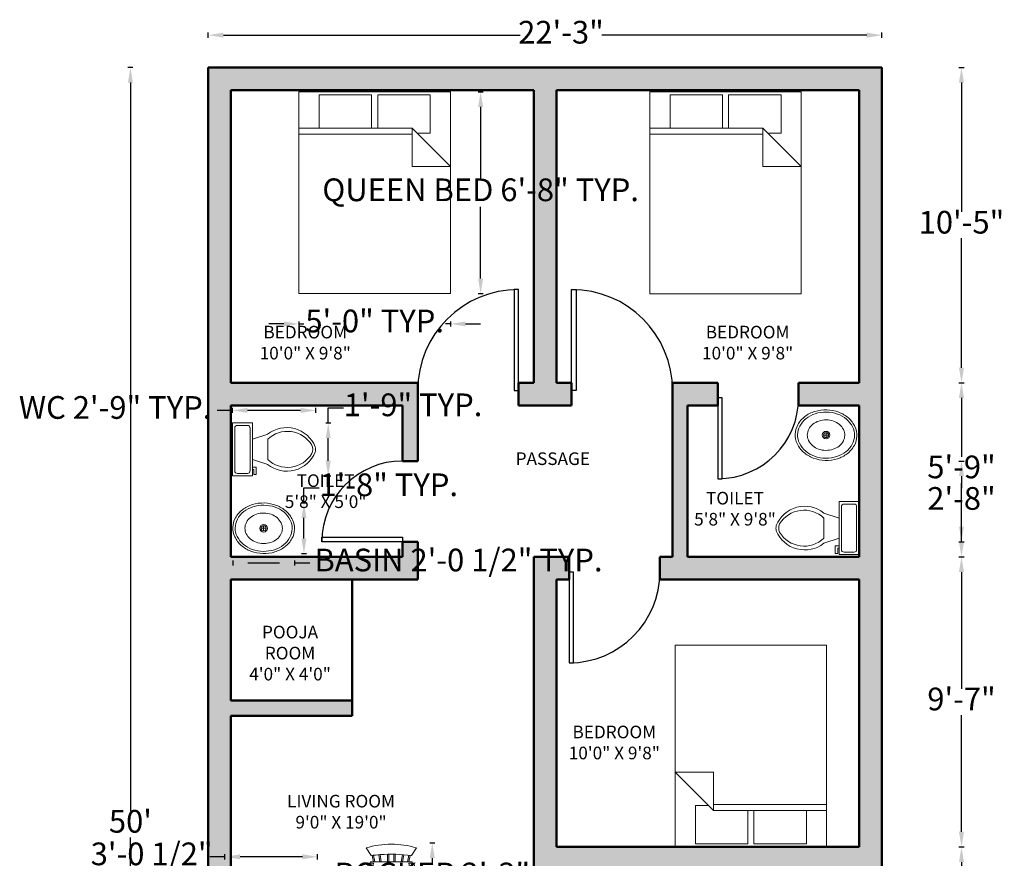
# Model space of a CAD drawing. Units: inches. Extents: x -31 to 401, y -19 to 637.
# Tile 2 of 2: x -31 to 359, y 305 to 637. Entities that reach past the tile are written whole.
import ezdxf

# ---------------------------------------------------------------- set-up
doc = ezdxf.new("R2010")
doc.units = ezdxf.units.IN
for name, color, linetype, lineweight in [('A-ANNO-DIMS', 2, 'Continuous', 18), ('A-AREA-IDEN', 7, 'Continuous', 25), ('A-DOOR', 4, 'Continuous', 25), ('A-FLOR-FIXT', 9, 'Continuous', 18), ('A-FURN', 8, 'Continuous', 18), ('A-WALL', 7, 'Continuous', 50), ('A-WALL-PATT', 252, 'Continuous', 13)]:
    doc.layers.add(name, color=color, linetype=linetype, lineweight=lineweight)
doc.styles.get("Standard").update_dxf_attribs({"font": 'arial.ttf'})
doc.dimstyles.new('ISO-25', dxfattribs={"dimtxt": 9, "dimasz": 6, "dimexe": 1, "dimexo": 2, "dimtad": 0, "dimtih": 1, "dimtoh": 1, "dimdec": 1, "dimlunit": 3, "dimtxsty": 'Standard', "dimcen": 2.5, "dimadec": 0, "dimazin": 0, "dimtfac": 1, "dimtdec": 1, "dimtmove": 0, "dimatfit": 3, "dimfxl": 1, "dimfxlon": 1, "dimarcsym": 0})

# ---------------------------------------------------------------- blocks, each defined once
blk = doc.blocks.new('*U6')
for p, q in [((0, 0), (0, 6)), ((36, 0), (36, 6))]:
    blk.add_line(p, q)
blk.add_lwpolyline([(0, 0), (0, -36), (1.75, -36), (1.75, 0)], close=True)
blk.add_arc((0, 0), 36, 270, 0)
blk = doc.blocks.new('*U4')
for p, q in [((0, 0), (0, -6)), ((-40, 0), (-40, -6))]:
    blk.add_line(p, q)
blk.add_lwpolyline([(0, 0), (0, 40), (-1.75, 40), (-1.75, 0)], close=True)
blk.add_arc((0, 0), 40, 90, 180)
blk = doc.blocks.new('*U10')
for p, q in [((0, 0), (0, -6)), ((32, 0), (32, -6))]:
    blk.add_line(p, q)
blk.add_lwpolyline([(0, 0), (0, 32), (1.75, 32), (1.75, 0)], close=True)
blk.add_arc((0, 0), 32, 0, 90)
blk = doc.blocks.new('*U3')
for p, q in [((0, 0), (0, -6)), ((40, 0), (40, -6))]:
    blk.add_line(p, q)
blk.add_lwpolyline([(0, 0), (0, 40), (1.75, 40), (1.75, 0)], close=True)
blk.add_arc((0, 0), 40, 0, 90)
blk = doc.blocks.new('*U5')
for p, q in [((0, 0), (0, 6)), ((32, 0), (32, 6))]:
    blk.add_line(p, q)
blk.add_lwpolyline([(0, 0), (0, -32), (1.75, -32), (1.75, 0)], close=True)
blk.add_arc((0, 0), 32, 270, 0)
blk = doc.blocks.new('Bed - Queen')
for p, q in [((0, -80.00003), (0, 0)), ((0, 0), (59.99999, 0)), ((59.99999, 0), (59.99999, -80.00003)), ((7.99999, -1.2), (28.79998, -1.2)), ((7.99999, -14.4), (7.99999, -1.2)), ((28.79998, -1.2), (28.79998, -14.4)), ((31.19999, -1.2), (51.99999, -1.2)), ((31.19999, -14.4), (31.19999, -1.2)), ((51.99999, -1.2), (51.99999, -16.4)), ((0, -14.4), (44.8, -14.4)), ((59.99999, -29.6), (44.8, -14.4)), ((44.8, -14.4), (44.8, -29.6)), ((44.8, -16.8), (0, -16.8)), ((51.99999, -16.4), (46.79936, -16.4)), ((44.8, -29.6), (59.99999, -29.6)), ((59.99999, -80.00003), (0, -80.00003))]:
    blk.add_line(p, q)
blk = doc.blocks.new('Chair - Rocking')
for p, q in [((-8, -4.5), (-10, -1.5)), ((8, -4.5), (10, -1.5)), ((-9, -7.5), (-12, -18.49999)), ((-7, -7.5), (-9, -7.5)), ((-9, -18.49999), (-7, -7.5)), ((-8.23428, -6.99939), (-8.3093, -7.47958)), ((-8.23041, -7), (8.23915, -7)), ((-7.5, -4.5), (-7, -7)), ((-6.5, -7), (-7.02225, -4.43)), ((-4.5, -7), (-4.96674, -4.19951)), ((-4, -7), (-4.40532, -4.16272)), ((-1.5, -4.05012), (-1.5, -7)), ((-1, -7), (-1, -4.05012)), ((1, -7), (1, -4.04655)), ((1.5, -4.05012), (1.5, -7)), ((4, -7), (4.40187, -4.18694)), ((4.5, -7), (4.96761, -4.19437)), ((6.5, -7), (7, -4.4057)), ((7.5, -4.5), (7, -7)), ((7, -7.5), (9, -7.5)), ((9, -18.49999), (7, -7.5)), ((8.31071, -7.48854), (8.23449, -7.00073)), ((9, -7.5), (12, -18.49999)), ((-10.36644, -20.64523), (-10.5, -21.49999)), ((-9, -22.49999), (-9.5, -26.49999)), ((0, -22.49999), (-9.5, -22.49999)), ((-8, -26.49999), (-7.5, -22.49999)), ((0, -22.49999), (9.5, -22.49999)), ((8, -26.49999), (7.5, -22.49999)), ((9, -22.49999), (9.5, -26.49999)), ((10.5, -21.49999), (10.3575, -20.58798)), ((-9.5, -26.49999), (-8, -26.49999)), ((9.5, -26.49999), (8, -26.49999))]:
    blk.add_line(p, q)
for centre, radius, start, end in [((0, -34.08333), 34.08333, 72.93847, 107.0615), ((0, -68.25004), 64.25, 93.92211, 97.15267), ((0, -68.25004), 64.25, 82.84733, 93.92211), ((-10.5, -18.99999), 1.58114, 161.5651, 18.43495), ((10.5, -18.99999), 1.58114, 161.5651, 18.43495), ((-9.5, -21.49999), 1, 180, 270), ((9.5, -21.49999), 1, 270, 0)]:
    blk.add_arc(centre, radius, start, end)
blk = doc.blocks.new('Toilet - top')
for p, q in [((9.5, -6), (9.5, -2)), ((-10, -8.5), (-8, -8.5)), ((-10, -9.5), (-10, -8.5)), ((-7, -9.5), (-10, -9.5)), ((-8, -8.5), (-8, -8)), ((-7, -8), (-7, -9.5)), ((-4, -8), (-6, -14)), ((4, -8), (6, -14)), ((4, -14), (-4, -14))]:
    blk.add_line(p, q)
blk.add_lwpolyline([(10.5, -8), (10.5, 0), (-10.5, 0), (-10.5, -8)], close=True)
for points in [[(-9.5, -2), (-9.5, -6)], [(8.5, -1), (-8.5, -1)], [(-8.5, -7), (8.5, -7)]]:
    blk.add_lwpolyline(points)
for centre, radius, start, end in [((-8.62, -1.88), 0.884, 81.8699, 188.1301), ((8.62, -1.88), 0.884, 351.8699, 98.1301), ((-8.62, -6.12), 0.884, 171.8699, 278.1301), ((8.62, -6.12), 0.884, 261.8699, 8.1301), ((3.52, -21.58), 12.17, 141.4691, 247.9714), ((4.2, -21.82), 11.33, 136.3677, 238.9468), ((-3.52, -21.58), 12.17, 292.0284, 38.5307), ((-4.2, -21.82), 11.33, 301.053, 43.6321), ((0, -27.88), 4, 245.7318, 294.2682), ((0, -29), 4, 254.8605, 285.1395)]:
    blk.add_arc(centre, radius, start, end)
blk = doc.blocks.new('Sink - Oval top')
for p, q in [((-1, 0), (1, 0)), ((0, 1), (0, -1))]:
    blk.add_line(p, q)
for points in [[(-12.23, 0.39, 0.117634), (-11.46, -3.36, 0.104469), (-8.88, -6.8, 0.090016), (-5.08, -9.07, 0.08192), (-0.32, -10.02, 0.08192), (4.49, -9.38, 0.090016), (8.42, -7.36, 0.104469), (11.22, -4.09, 0.117634), (12.23, -0.39, 0.117634), (11.46, 3.36, 0.104469), (8.88, 6.8, 0.090016), (5.08, 9.07, 0.08192), (0.32, 10.02, 0.08192), (-4.49, 9.38, 0.090016), (-8.42, 7.36, 0.104469), (-11.22, 4.09, 0.117634)], [(-11.29, 0.16, 0.118622), (-10.52, -3.25, 0.104678), (-8.07, -6.36, 0.089562), (-4.54, -8.37, 0.081185), (-0.13, -9.15, 0.081185), (4.3, -8.49, 0.089562), (7.89, -6.58, 0.104678), (10.42, -3.55, 0.118622), (11.29, -0.16, 0.118622), (10.52, 3.25, 0.104678), (8.07, 6.36, 0.089562), (4.54, 8.37, 0.081185), (0.13, 9.15, 0.081185), (-4.3, 8.49, 0.089562), (-7.89, 6.58, 0.104678), (-10.42, 3.55, 0.118622)], [(-7.42, 0.08, 0.118283), (-6.91, -2.17, 0.104607), (-5.29, -4.21, 0.089718), (-2.97, -5.53, 0.081436), (-0.07, -6.04, 0.081436), (2.84, -5.59, 0.089718), (5.2, -4.33, 0.104607), (6.86, -2.32, 0.118283), (7.42, -0.08, 0.118283), (6.91, 2.17, 0.104607), (5.29, 4.21, 0.089718), (2.97, 5.53, 0.081436), (0.07, 6.04, 0.081436), (-2.84, 5.59, 0.089718), (-5.2, 4.33, 0.104607), (-6.86, 2.32, 0.118283)]]:
    blk.add_lwpolyline(points, format="xyb", close=True)
for radius in [1.5, 1]:
    blk.add_circle((0, 0), radius)
blk = doc.blocks.new('*D20')
at = {"layer": 'A-ANNO-DIMS', "color": 0, "lineweight": -2, "transparency": 16777216}
for p, q in [((13.91, 618.38), (11.91, 618.38)), ((12.91, 612.38), (12.91, 323.6)), ((12.91, 24.38), (12.91, 313.16)), ((13.91, 18.38), (11.91, 18.38))]:
    blk.add_line(p, q, dxfattribs=at)
at = {"layer": 'A-ANNO-DIMS', "color": 0, "transparency": 16777216}
for points in [[(11.91, 612.38), (13.91, 612.38), (12.91, 618.38)], [(11.91, 24.38), (13.91, 24.38), (12.91, 18.38)]]:
    blk.add_solid(points, dxfattribs=at)
at = {"layer": 'Defpoints', "color": 0, "transparency": 16777216}
for p in [(43.78, 618.38), (12.91, 18.38), (43.78, 18.38)]:
    blk.add_point(p, dxfattribs=at)
at = {"layer": 'A-ANNO-DIMS', "color": 0, "transparency": 16777216, "insert": (12.91, 318.38), "char_height": 9, "attachment_point": 5}
blk.add_mtext("50'", dxfattribs=at)
blk = doc.blocks.new('*D21')
at = {"layer": 'A-ANNO-DIMS', "color": 0, "lineweight": -2, "transparency": 16777216}
for p, q in [((43.78, 630.2), (43.78, 632.2)), ((49.78, 631.2), (167.43, 631.2)), ((304.78, 631.2), (199.75, 631.2)), ((310.78, 630.2), (310.78, 632.2))]:
    blk.add_line(p, q, dxfattribs=at)
at = {"layer": 'A-ANNO-DIMS', "color": 0, "transparency": 16777216}
for points in [[(49.78, 632.2), (49.78, 630.2), (43.78, 631.2)], [(304.78, 632.2), (304.78, 630.2), (310.78, 631.2)]]:
    blk.add_solid(points, dxfattribs=at)
at = {"layer": 'Defpoints', "color": 0, "transparency": 16777216}
for p in [(310.78, 631.2), (43.78, 618.38), (310.78, 618.38)]:
    blk.add_point(p, dxfattribs=at)
at = {"layer": 'A-ANNO-DIMS', "color": 0, "transparency": 16777216, "insert": (183.59, 631.2), "char_height": 9, "attachment_point": 5}
blk.add_mtext('22\'-3"', dxfattribs=at)
blk = doc.blocks.new('*D22')
at = {"layer": 'A-ANNO-DIMS', "color": 0, "lineweight": -2, "transparency": 16777216}
for p, q in [((150.73, 608.73), (152.73, 608.73)), ((151.73, 602.73), (151.73, 574.28)), ((151.73, 534.73), (151.73, 563.17)), ((150.73, 528.73), (152.73, 528.73))]:
    blk.add_line(p, q, dxfattribs=at)
at = {"layer": 'A-ANNO-DIMS', "color": 0, "transparency": 16777216}
for points in [[(150.73, 602.73), (152.73, 602.73), (151.73, 608.73)], [(150.73, 534.73), (152.73, 534.73), (151.73, 528.73)]]:
    blk.add_solid(points, dxfattribs=at)
at = {"layer": 'Defpoints', "color": 0, "transparency": 16777216}
for p in [(139.73, 608.73), (151.73, 608.73), (139.73, 528.73)]:
    blk.add_point(p, dxfattribs=at)
at = {"layer": 'A-ANNO-DIMS', "color": 0, "transparency": 16777216, "insert": (151.73, 568.73), "char_height": 9, "attachment_point": 5}
blk.add_mtext('QUEEN BED 6\'-8" TYP.', dxfattribs=at)
blk = doc.blocks.new('*D23')
at = {"layer": 'A-ANNO-DIMS', "color": 0, "lineweight": -2, "transparency": 16777216}
for p, q in [((73.73, 516.73), (67.73, 516.73)), ((79.73, 517.73), (79.73, 515.73)), ((79.73, 516.73), (81.67, 516.73)), ((139.73, 516.73), (137.78, 516.73)), ((139.73, 517.73), (139.73, 515.73)), ((145.73, 516.73), (151.73, 516.73))]:
    blk.add_line(p, q, dxfattribs=at)
at = {"layer": 'A-ANNO-DIMS', "color": 0, "transparency": 16777216}
for points in [[(73.73, 517.73), (73.73, 515.73), (79.73, 516.73)], [(145.73, 517.73), (145.73, 515.73), (139.73, 516.73)]]:
    blk.add_solid(points, dxfattribs=at)
at = {"layer": 'Defpoints', "color": 0, "transparency": 16777216}
for p in [(79.73, 528.73), (139.73, 528.73), (139.73, 516.73)]:
    blk.add_point(p, dxfattribs=at)
at = {"layer": 'A-ANNO-DIMS', "color": 0, "transparency": 16777216, "insert": (109.73, 516.73), "char_height": 9, "attachment_point": 5}
blk.add_mtext('5\'-0" TYP.', dxfattribs=at)
blk = doc.blocks.new('*D24')
at = {"layer": 'A-ANNO-DIMS', "color": 0, "lineweight": -2, "transparency": 16777216}
for p, q in [((53.32, 482.44), (47.32, 482.44)), ((53.32, 481.44), (53.32, 483.44)), ((80.36, 482.44), (59.32, 482.44)), ((86.36, 481.44), (86.36, 483.44))]:
    blk.add_line(p, q, dxfattribs=at)
at = {"layer": 'A-ANNO-DIMS', "color": 0, "transparency": 16777216}
for points in [[(59.32, 483.44), (59.32, 481.44), (53.32, 482.44)], [(80.36, 483.44), (80.36, 481.44), (86.36, 482.44)]]:
    blk.add_solid(points, dxfattribs=at)
at = {"layer": 'Defpoints', "color": 0, "transparency": 16777216}
for p in [(53.32, 482.44), (53.32, 477.49), (86.36, 477.49)]:
    blk.add_point(p, dxfattribs=at)
at = {"layer": 'A-ANNO-DIMS', "color": 0, "transparency": 16777216, "insert": (6.86, 482.44), "char_height": 9, "attachment_point": 5}
blk.add_mtext('WC 2\'-9" TYP.', dxfattribs=at)
blk = doc.blocks.new('*D25')
at = {"layer": 'A-ANNO-DIMS', "color": 0, "lineweight": -2, "transparency": 16777216}
for p, q in [((91.32, 477.49), (91.32, 483.49)), ((91.32, 483.49), (97.32, 483.49)), ((90.32, 477.49), (92.32, 477.49)), ((91.32, 462.49), (91.32, 471.49)), ((90.32, 456.49), (92.32, 456.49))]:
    blk.add_line(p, q, dxfattribs=at)
at = {"layer": 'A-ANNO-DIMS', "color": 0, "transparency": 16777216}
for points in [[(90.32, 471.49), (92.32, 471.49), (91.32, 477.49)], [(90.32, 462.49), (92.32, 462.49), (91.32, 456.49)]]:
    blk.add_solid(points, dxfattribs=at)
at = {"layer": 'Defpoints', "color": 0, "transparency": 16777216}
for p in [(86.36, 477.49), (91.32, 477.49), (86.36, 456.49)]:
    blk.add_point(p, dxfattribs=at)
at = {"layer": 'A-ANNO-DIMS', "color": 0, "transparency": 16777216, "insert": (124.95, 483.49), "char_height": 9, "attachment_point": 5}
blk.add_mtext('1\'-9" TYP.', dxfattribs=at)
blk = doc.blocks.new('*D26')
at = {"layer": 'A-ANNO-DIMS', "color": 0, "lineweight": -2, "transparency": 16777216}
for p, q in [((53.46, 422.97), (53.46, 420.97)), ((59.46, 421.97), (72.01, 421.97)), ((78.01, 422.97), (78.01, 420.97)), ((78.01, 421.97), (84.01, 421.97))]:
    blk.add_line(p, q, dxfattribs=at)
at = {"layer": 'A-ANNO-DIMS', "color": 0, "transparency": 16777216}
for points in [[(59.46, 422.97), (59.46, 420.97), (53.46, 421.97)], [(72.01, 422.97), (72.01, 420.97), (78.01, 421.97)]]:
    blk.add_solid(points, dxfattribs=at)
at = {"layer": 'Defpoints', "color": 0, "transparency": 16777216}
for p in [(53.46, 425.65), (78.01, 425.65), (78.01, 421.97)]:
    blk.add_point(p, dxfattribs=at)
at = {"layer": 'A-ANNO-DIMS', "color": 0, "transparency": 16777216, "insert": (142.96, 421.97), "char_height": 9, "attachment_point": 5}
blk.add_mtext('BASIN 2\'-0 1/2" TYP.', dxfattribs=at)
blk = doc.blocks.new('*D27')
at = {"layer": 'A-ANNO-DIMS', "color": 0, "lineweight": -2, "transparency": 16777216}
for p, q in [((81.69, 445.79), (81.69, 451.79)), ((81.69, 451.79), (87.69, 451.79)), ((80.69, 445.79), (82.69, 445.79)), ((81.69, 431.65), (81.69, 439.79)), ((80.69, 425.65), (82.69, 425.65))]:
    blk.add_line(p, q, dxfattribs=at)
at = {"layer": 'A-ANNO-DIMS', "color": 0, "transparency": 16777216}
for points in [[(80.69, 439.79), (82.69, 439.79), (81.69, 445.79)], [(80.69, 431.65), (82.69, 431.65), (81.69, 425.65)]]:
    blk.add_solid(points, dxfattribs=at)
at = {"layer": 'Defpoints', "color": 0, "transparency": 16777216}
for p in [(78.01, 445.79), (81.69, 445.79), (78.01, 425.65)]:
    blk.add_point(p, dxfattribs=at)
at = {"layer": 'A-ANNO-DIMS', "color": 0, "transparency": 16777216, "insert": (115.32, 451.79), "char_height": 9, "attachment_point": 5}
blk.add_mtext('1\'-8" TYP.', dxfattribs=at)
blk = doc.blocks.new('*D29')
at = {"layer": 'A-ANNO-DIMS', "color": 0, "lineweight": -2, "transparency": 16777216}
for p, q in [((50.4, 305.47), (44.4, 305.47)), ((50.4, 304.47), (50.4, 306.47)), ((81.07, 305.47), (56.4, 305.47)), ((87.07, 304.47), (87.07, 306.47))]:
    blk.add_line(p, q, dxfattribs=at)
at = {"layer": 'A-ANNO-DIMS', "color": 0, "transparency": 16777216}
for points in [[(56.4, 306.47), (56.4, 304.47), (50.4, 305.47)], [(81.07, 306.47), (81.07, 304.47), (87.07, 305.47)]]:
    blk.add_solid(points, dxfattribs=at)
at = {"layer": 'Defpoints', "color": 0, "transparency": 16777216}
for p in [(50.4, 305.47), (50.4, 292.87), (87.07, 292.87)]:
    blk.add_point(p, dxfattribs=at)
at = {"layer": 'A-ANNO-DIMS', "color": 0, "transparency": 16777216, "insert": (21.33, 305.47), "char_height": 9, "attachment_point": 5}
blk.add_mtext('3\'-0 1/2"', dxfattribs=at)
blk = doc.blocks.new('*D30')
at = {"layer": 'A-ANNO-DIMS', "color": 0, "lineweight": -2, "transparency": 16777216}
for p, q in [((131.57, 310.98), (133.57, 310.98)), ((132.57, 304.98), (132.57, 302.76)), ((132.57, 289.98), (132.57, 292.19)), ((131.57, 283.98), (133.57, 283.98))]:
    blk.add_line(p, q, dxfattribs=at)
at = {"layer": 'A-ANNO-DIMS', "color": 0, "transparency": 16777216}
for points in [[(131.57, 304.98), (133.57, 304.98), (132.57, 310.98)], [(131.57, 289.98), (133.57, 289.98), (132.57, 283.98)]]:
    blk.add_solid(points, dxfattribs=at)
at = {"layer": 'Defpoints', "color": 0, "transparency": 16777216}
for p in [(128.52, 310.98), (132.57, 310.98), (128.52, 283.98)]:
    blk.add_point(p, dxfattribs=at)
at = {"layer": 'A-ANNO-DIMS', "color": 0, "transparency": 16777216, "insert": (132.57, 297.48), "char_height": 9, "attachment_point": 5}
blk.add_mtext('ROCKER 2\'-3"', dxfattribs=at)
blk = doc.blocks.new('*D45')
at = {"layer": 'A-ANNO-DIMS', "color": 0, "lineweight": -2, "transparency": 16777216}
for p, q in [((341.33, 309.38), (343.33, 309.38)), ((342.33, 303.38), (342.33, 238.1)), ((342.33, 162.38), (342.33, 227.66)), ((341.33, 156.38), (343.33, 156.38))]:
    blk.add_line(p, q, dxfattribs=at)
at = {"layer": 'A-ANNO-DIMS', "color": 0, "transparency": 16777216}
for points in [[(341.33, 303.38), (343.33, 303.38), (342.33, 309.38)], [(341.33, 162.38), (343.33, 162.38), (342.33, 156.38)]]:
    blk.add_solid(points, dxfattribs=at)
at = {"layer": 'Defpoints', "color": 0, "transparency": 16777216}
for p in [(301.78, 309.38), (342.33, 309.38), (301.78, 156.38)]:
    blk.add_point(p, dxfattribs=at)
at = {"layer": 'A-ANNO-DIMS', "color": 0, "transparency": 16777216, "insert": (342.33, 232.88), "char_height": 9, "attachment_point": 5}
blk.add_mtext('12\'-9"', dxfattribs=at)
blk = doc.blocks.new('*D46')
at = {"layer": 'A-ANNO-DIMS', "color": 0, "lineweight": -2, "transparency": 16777216}
for p, q in [((341.33, 424.38), (343.33, 424.38)), ((342.33, 418.38), (342.33, 372.1)), ((342.33, 315.38), (342.33, 361.66)), ((341.33, 309.38), (343.33, 309.38))]:
    blk.add_line(p, q, dxfattribs=at)
at = {"layer": 'A-ANNO-DIMS', "color": 0, "transparency": 16777216}
for points in [[(341.33, 418.38), (343.33, 418.38), (342.33, 424.38)], [(341.33, 315.38), (343.33, 315.38), (342.33, 309.38)]]:
    blk.add_solid(points, dxfattribs=at)
at = {"layer": 'Defpoints', "color": 0, "transparency": 16777216}
for p in [(301.78, 424.38), (342.33, 424.38), (301.78, 309.38)]:
    blk.add_point(p, dxfattribs=at)
at = {"layer": 'A-ANNO-DIMS', "color": 0, "transparency": 16777216, "insert": (342.33, 366.88), "char_height": 9, "attachment_point": 5}
blk.add_mtext('9\'-7"', dxfattribs=at)
blk = doc.blocks.new('*D47')
at = {"layer": 'A-ANNO-DIMS', "color": 0, "lineweight": -2, "transparency": 16777216}
for p, q in [((341.33, 493.38), (343.33, 493.38)), ((342.33, 487.38), (342.33, 464.1)), ((342.33, 430.38), (342.33, 453.66)), ((341.33, 424.38), (343.33, 424.38))]:
    blk.add_line(p, q, dxfattribs=at)
at = {"layer": 'A-ANNO-DIMS', "color": 0, "transparency": 16777216}
for points in [[(341.33, 487.38), (343.33, 487.38), (342.33, 493.38)], [(341.33, 430.38), (343.33, 430.38), (342.33, 424.38)]]:
    blk.add_solid(points, dxfattribs=at)
at = {"layer": 'Defpoints', "color": 0, "transparency": 16777216}
for p in [(301.78, 493.38), (342.33, 493.38), (301.78, 424.38)]:
    blk.add_point(p, dxfattribs=at)
at = {"layer": 'A-ANNO-DIMS', "color": 0, "transparency": 16777216, "insert": (342.33, 458.88), "char_height": 9, "attachment_point": 5}
blk.add_mtext('5\'-9"', dxfattribs=at)
blk = doc.blocks.new('*D48')
at = {"layer": 'A-ANNO-DIMS', "color": 0, "lineweight": -2, "transparency": 16777216}
for p, q in [((341.33, 618.38), (343.33, 618.38)), ((342.33, 612.38), (342.33, 561.1)), ((342.33, 499.38), (342.33, 550.66)), ((341.33, 493.38), (343.33, 493.38))]:
    blk.add_line(p, q, dxfattribs=at)
at = {"layer": 'A-ANNO-DIMS', "color": 0, "transparency": 16777216}
for points in [[(341.33, 612.38), (343.33, 612.38), (342.33, 618.38)], [(341.33, 499.38), (343.33, 499.38), (342.33, 493.38)]]:
    blk.add_solid(points, dxfattribs=at)
at = {"layer": 'Defpoints', "color": 0, "transparency": 16777216}
for p in [(310.78, 618.38), (342.33, 618.38), (301.78, 493.38)]:
    blk.add_point(p, dxfattribs=at)
at = {"layer": 'A-ANNO-DIMS', "color": 0, "transparency": 16777216, "insert": (342.33, 555.88), "char_height": 9, "attachment_point": 5}
blk.add_mtext('10\'-5"', dxfattribs=at)
blk = doc.blocks.new('*D49')
at = {"layer": 'A-ANNO-DIMS', "color": 0, "lineweight": -2, "transparency": 16777216}
for p, q in [((341.33, 462.38), (343.33, 462.38)), ((342.33, 456.38), (342.33, 451.6)), ((342.33, 436.38), (342.33, 441.16)), ((341.33, 430.38), (343.33, 430.38))]:
    blk.add_line(p, q, dxfattribs=at)
at = {"layer": 'A-ANNO-DIMS', "color": 0, "transparency": 16777216}
for points in [[(341.33, 456.38), (343.33, 456.38), (342.33, 462.38)], [(341.33, 436.38), (343.33, 436.38), (342.33, 430.38)]]:
    blk.add_solid(points, dxfattribs=at)
at = {"layer": 'Defpoints', "color": 0, "transparency": 16777216}
for p in [(126.78, 462.38), (342.33, 462.38), (126.78, 430.38)]:
    blk.add_point(p, dxfattribs=at)
at = {"layer": 'A-ANNO-DIMS', "color": 0, "transparency": 16777216, "insert": (342.33, 446.38), "char_height": 9, "attachment_point": 5}
blk.add_mtext('2\'-8"', dxfattribs=at)

msp = doc.modelspace()

# ---------------------------------------------------------------- hatches: boundary and pattern name
at = {"layer": 'A-WALL-PATT'}
h = msp.add_hatch(color=256, dxfattribs=at)
h.dxf.hatch_style = 1
h.paths.add_polyline_path([(310.78, 618.38), (43.78, 618.38), (43.78, 18.38), (58.78, 18.38), (58.78, 24.38), (58.78, 27.38), (52.78, 27.38), (52.78, 147.38), (130.78, 147.38), (130.78, 153.38), (130.78, 156.38), (52.78, 156.38), (52.78, 361.38), (100.78, 361.38), (100.78, 367.38), (52.78, 367.38), (52.78, 415.38), (126.78, 415.38), (126.78, 430.38), (120.78, 430.38), (120.78, 424.38), (52.78, 424.38), (52.78, 484.38), (120.78, 484.38), (120.78, 462.38), (126.78, 462.38), (126.78, 493.38), (52.78, 493.38), (52.78, 609.38), (172.78, 609.38), (172.78, 493.38), (166.78, 493.38), (166.78, 490.38), (166.78, 484.38), (187.81, 484.38), (187.81, 490.38), (187.81, 493.38), (181.78, 493.38), (181.78, 609.38), (301.78, 609.38), (301.78, 493.38), (277.78, 493.38), (277.78, 487.38), (277.78, 484.38), (301.78, 484.38), (301.78, 424.38), (233.78, 424.38), (233.78, 484.38), (245.78, 484.38), (245.78, 487.38), (245.78, 493.38), (227.78, 493.38), (227.78, 491.76, -0.008619), (227.81, 490.38), (227.81, 484.38), (227.78, 424.38), (222.78, 424.38), (222.78, 418.38), (222.78, 415.38), (301.78, 415.38), (301.78, 309.38), (181.78, 309.38), (181.78, 415.38), (186.78, 415.38), (186.78, 418.38), (186.78, 424.38), (172.78, 424.38), (172.78, 300.38), (301.78, 300.38), (301.78, 228.38), (219.84, 228.38), (219.84, 219.38), (301.78, 219.38), (301.78, 156.38), (181.78, 156.38), (181.78, 219.38), (181.78, 268.42), (172.78, 268.42), (172.78, 156.38), (166.78, 156.38), (166.78, 153.38), (166.78, 147.38), (301.78, 147.38), (301.78, 27.38), (118.78, 27.38), (118.78, 24.38), (118.78, 18.38), (310.78, 18.38)])

# ---------------------------------------------------------------- linework, layer by layer
at = {"layer": 'A-WALL'}
for p, q in [((310.78, 618.38), (43.78, 618.38)), ((43.78, 618.38), (43.78, 18.38)), ((310.78, 18.38), (310.78, 618.38)), ((52.78, 609.38), (52.78, 493.38)), ((172.78, 609.38), (52.78, 609.38)), ((172.78, 609.38), (172.78, 493.38)), ((301.78, 609.38), (181.78, 609.38)), ((181.78, 493.38), (181.78, 609.38)), ((301.78, 493.38), (301.78, 609.38)), ((126.78, 493.38), (52.78, 493.38)), ((126.78, 493.38), (126.78, 462.38)), ((172.78, 493.38), (166.78, 493.38)), ((166.78, 493.38), (166.78, 484.38)), ((187.81, 493.38), (181.78, 493.38)), ((187.81, 493.38), (187.81, 484.38)), ((227.78, 424.38), (227.78, 493.38)), ((245.78, 493.38), (227.78, 493.38)), ((245.78, 484.38), (245.78, 493.38)), ((301.78, 493.38), (277.78, 493.38)), ((277.78, 484.38), (277.78, 493.38)), ((52.78, 484.38), (52.78, 424.38)), ((120.78, 484.38), (52.78, 484.38)), ((120.78, 484.38), (120.78, 462.38)), ((187.81, 484.38), (166.78, 484.38)), ((233.78, 424.38), (233.78, 484.38)), ((245.78, 484.38), (233.78, 484.38)), ((301.78, 484.38), (277.78, 484.38)), ((301.78, 424.38), (301.78, 484.38)), ((120.78, 462.38), (126.78, 462.38)), ((120.78, 430.38), (126.78, 430.38)), ((120.78, 430.38), (120.78, 424.38)), ((126.78, 430.38), (126.78, 415.38)), ((120.78, 424.38), (52.78, 424.38)), ((186.78, 424.38), (172.78, 424.38)), ((172.78, 300.38), (172.78, 424.38)), ((186.78, 415.38), (186.78, 424.38)), ((227.78, 424.38), (222.78, 424.38)), ((222.78, 415.38), (222.78, 424.38)), ((301.78, 424.38), (233.78, 424.38)), ((126.78, 415.38), (52.78, 415.38)), ((52.78, 415.38), (52.78, 367.38)), ((100.78, 415.38), (100.78, 361.38)), ((181.78, 309.38), (181.78, 415.38)), ((186.78, 415.38), (181.78, 415.38)), ((301.78, 415.38), (222.78, 415.38)), ((301.78, 309.38), (301.78, 415.38)), ((100.78, 367.38), (52.78, 367.38)), ((100.78, 361.38), (52.78, 361.38)), ((52.78, 361.38), (52.78, 156.38)), ((181.78, 309.38), (301.78, 309.38))]:
    msp.add_line(p, q, dxfattribs=at)

# ---------------------------------------------------------------- block references
at = {"layer": 'A-DOOR'}
for name, p in [('*U4', (166.78, 490.38)), ('*U3', (187.81, 490.38)), ('*U5', (245.78, 487.38)), ('*U6', (186.78, 418.38))]:
    msp.add_blockref(name, p, dxfattribs=at)
at = {"layer": 'A-DOOR', "rotation": 90}
msp.add_blockref('*U10', (120.78, 430.38), dxfattribs=at)
at = {"layer": 'A-FLOR-FIXT'}
for p in [(288.64, 472.64), (65.73, 435.72)]:
    msp.add_blockref('Sink - Oval top', p, dxfattribs=at)
at = {"layer": 'A-FLOR-FIXT', "rotation": 90}
msp.add_blockref('Toilet - top', (53.32, 466.99), dxfattribs=at)
at = {"layer": 'A-FLOR-FIXT', "xscale": -1, "rotation": 270}
msp.add_blockref('Toilet - top', (301.78, 435.77), dxfattribs=at)
at = {"layer": 'A-FURN'}
for name, p in [('Bed - Queen', (79.73, 608.73)), ('Bed - Queen', (218.81, 608.7)), ('Chair - Rocking', (116.3, 310.48))]:
    msp.add_blockref(name, p, dxfattribs=at)
at = {"layer": 'A-FURN', "rotation": 180}
msp.add_blockref('Bed - Queen', (288.85, 309.38), dxfattribs=at)

# ---------------------------------------------------------------- texts
at = {"layer": 'A-AREA-IDEN', "char_height": 5, "attachment_point": 1}
for s, width, insert in [('\\pxqc;BEDROOM\\P10\'0" X 9\'8"', 40.9025, (61.77, 515.98)), ('\\pxqc;BEDROOM\\P10\'0" X 9\'8"', 40.9025, (237.11, 515.98)), ('\\pxqc;PASSAGE', 40.9025, (159.9, 465.8)), ('\\pxqc;TOILET\\P5\'8" X 5\'0"', 40.9025, (69.84, 457.09)), ('\\pxqc;TOILET\\P5\'8" X 9\'8"', 40.9025, (232.1, 450.15)), ('\\pxqc;POOJA\\PROOM\\P4\'0" X 4\'0"', 40.9025, (55.74, 397.07)), ('\\pxqc;BEDROOM\\P10\'0" X 9\'8"', 40.9025, (184.28, 357.46)), ('\\pxqc;LIVING ROOM\\P9\'0" X 19\'0"', 50.39, (71.21, 330.03))]:
    msp.add_mtext_dynamic_manual_height_columns(s, width=width, gutter_width=12.5, heights=[0], dxfattribs=dict(at, insert=insert))

# ---------------------------------------------------------------- dimensions: what is measured, and where the dimension line sits
at = {"layer": 'A-ANNO-DIMS'}
dim = msp.add_linear_dim(base=(310.78, 631.2), p1=(43.78, 618.38), p2=(310.78, 618.38), dimstyle='ISO-25', override={"dimclrd": 0, "dimclre": 0, "dimclrt": 0}, dxfattribs=at)
dim.commit()
dim.dimension.update_dxf_attribs({"geometry": '*D21', "text_midpoint": (183.59, 631.2), "dimtype": 160})
for base, p1, p2, angle, override, picture, middle in [((12.91, 18.38), (43.78, 618.38), (43.78, 18.38), 90, {"dimclrd": 0, "dimclre": 0, "dimclrt": 0}, '*D20', (12.91, 318.38)), ((342.33, 618.38), (301.78, 493.38), (310.78, 618.38), 90, {"dimdec": 1, "dimlfac": 1, "dimrnd": 0, "dimzin": 1, "dimdsep": 46, "dimlunit": 4, "dimfrac": 2}, '*D48', (342.33, 555.88)), ((342.33, 493.38), (301.78, 424.38), (301.78, 493.38), 90, {"dimdec": 1, "dimlfac": 1, "dimrnd": 0, "dimzin": 1, "dimdsep": 46, "dimlunit": 4, "dimfrac": 2}, '*D47', (342.33, 458.88)), ((342.33, 462.38), (126.78, 430.38), (126.78, 462.38), 90, {"dimdec": 1, "dimlfac": 1, "dimrnd": 0, "dimzin": 1, "dimdsep": 46, "dimlunit": 4, "dimfrac": 2}, '*D49', (342.33, 446.38)), ((342.33, 424.38), (301.78, 309.38), (301.78, 424.38), 90, {"dimdec": 1, "dimlfac": 1, "dimrnd": 0, "dimzin": 1, "dimdsep": 46, "dimlunit": 4, "dimfrac": 2}, '*D46', (342.33, 366.88)), ((50.4, 305.47), (87.07, 292.87), (50.4, 292.87), 180, {"dimdec": 1, "dimlfac": 1, "dimrnd": 0, "dimzin": 1, "dimdsep": 46, "dimlunit": 4, "dimfrac": 2}, '*D29', (21.33, 305.47)), ((342.33, 309.38), (301.78, 156.38), (301.78, 309.38), 90, {"dimdec": 1, "dimlfac": 1, "dimrnd": 0, "dimzin": 1, "dimdsep": 46, "dimlunit": 4, "dimfrac": 2}, '*D45', (342.33, 232.88))]:
    dim = msp.add_linear_dim(base=base, p1=p1, p2=p2, angle=angle, dimstyle='ISO-25', override=override, dxfattribs=at)
    dim.commit()
    dim.dimension.update_dxf_attribs({"geometry": picture, "text_midpoint": middle})
for base, p1, p2, angle, text, picture, middle in [((151.73, 608.73), (139.73, 528.73), (139.73, 608.73), 90, 'QUEEN BED <> TYP.', '*D22', (151.73, 568.73)), ((53.32, 482.44), (86.36, 477.49), (53.32, 477.49), 180, 'WC <> TYP.', '*D24', (6.86, 482.44)), ((91.32, 477.49), (86.36, 456.49), (86.36, 477.49), 90, '<> TYP.', '*D25', (124.95, 483.49)), ((81.69, 445.79), (78.01, 425.65), (78.01, 445.79), 90, '<> TYP.', '*D27', (115.32, 451.79)), ((132.57, 310.98), (128.52, 283.98), (128.52, 310.98), 90, 'ROCKER <>', '*D30', (132.57, 297.48))]:
    dim = msp.add_linear_dim(base=base, p1=p1, p2=p2, angle=angle, text=text, dimstyle='ISO-25', override={"dimdec": 1, "dimlfac": 1, "dimrnd": 0, "dimzin": 1, "dimdsep": 46, "dimlunit": 4, "dimfrac": 2}, dxfattribs=at)
    dim.commit()
    dim.dimension.update_dxf_attribs({"geometry": picture, "text_midpoint": middle})
for base, p1, p2, text, picture, middle in [((139.73, 516.73), (79.73, 528.73), (139.73, 528.73), '<> TYP.', '*D23', (109.73, 516.73)), ((78.0072, 421.9706), (53.4563, 425.6533), (78.0072, 425.6533), 'BASIN <> TYP.', '*D26', (142.9603, 421.9706))]:
    dim = msp.add_linear_dim(base=base, p1=p1, p2=p2, text=text, dimstyle='ISO-25', override={"dimdec": 1, "dimlfac": 1, "dimrnd": 0, "dimzin": 1, "dimdsep": 46, "dimlunit": 4, "dimfrac": 2}, dxfattribs=at)
    dim.commit()
    dim.dimension.update_dxf_attribs({"geometry": picture, "text_midpoint": middle})

doc.saveas('drawing.dxf')
